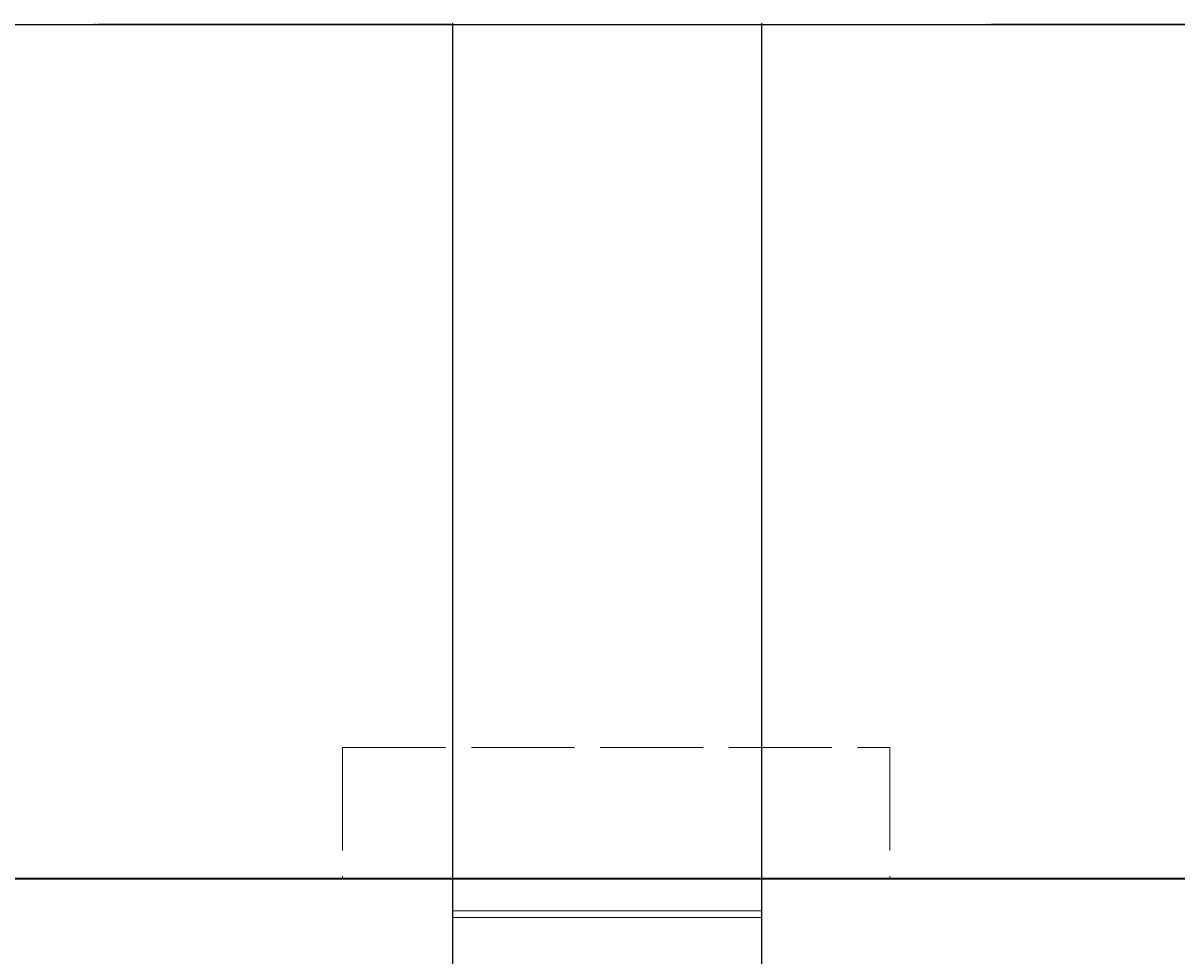
# Model space of a CAD drawing. Units: inches. Extents: x -61 to 1599, y -1316 to 257.
# Tile 153 of 204: x 406 to 540, y 149 to 257. Entities that reach past the tile are written whole.
import ezdxf

# ---------------------------------------------------------------- set-up
doc = ezdxf.new("R2010")
doc.units = ezdxf.units.IN
doc.header["$MEASUREMENT"] = 0
doc.linetypes.add('ACAD_ISO02W100', pattern=[15, 12, -3])
for name, color, linetype, lineweight in [('A-ANNO-DIMS', 2, 'Continuous', 18), ('A-FLOR-OVHD', 203, 'ACAD_ISO02W100', 13), ('WALLS', 4, 'Continuous', 35), ('WINDOWS', 220, 'Continuous', 18)]:
    doc.layers.add(name, color=color, linetype=linetype, lineweight=lineweight)
doc.styles.get("Standard").update_dxf_attribs({"font": 'arial.ttf'})
doc.dimstyles.get("Standard").update_dxf_attribs({"dimtxt": 0.18, "dimasz": 0.18, "dimexe": 0.18, "dimexo": 0.0625, "dimgap": 0.09, "dimtad": 0, "dimtih": 1, "dimtoh": 1, "dimdec": 0, "dimzin": 0, "dimdsep": 46, "dimlunit": 3, "dimtxsty": 'Standard', "dimcen": 0.09, "dimadec": 0, "dimazin": 0, "dimtfac": 1, "dimtdec": 0, "dimtofl": 0, "dimtmove": 0, "dimatfit": 3, "dimfxl": 1, "dimtolj": 1, "dimtzin": 0, "dimarcsym": 0})

# ---------------------------------------------------------------- blocks, each defined once
blk = doc.blocks.new('WIN-36IN')
for p, q in [((0, 4.5), (0, 9)), ((0, 9), (0, 0)), ((36, 9), (36, 0)), ((0, 5.26), (36, 5.26)), ((0, 4.5), (36, 4.5)), ((0, 4.5), (36, 4.5))]:
    blk.add_line(p, q)
blk = doc.blocks.new('*D686')
at = {"layer": 'A-ANNO-DIMS', "color": 0, "lineweight": -2, "transparency": 16777216}
for p, q in [((14.7, 157.74), (14.7, 257.46)), ((14.88, 257.28), (768.35, 257.28)), ((1522.52, 257.28), (769.05, 257.28)), ((1522.7, 157.74), (1522.7, 257.46))]:
    blk.add_line(p, q, dxfattribs=at)
at = {"layer": 'A-ANNO-DIMS', "color": 0, "transparency": 16777216}
for points in [[(14.88, 257.31), (14.88, 257.25), (14.7, 257.28)], [(1522.52, 257.31), (1522.52, 257.25), (1522.7, 257.28)]]:
    blk.add_solid(points, dxfattribs=at)
at = {"layer": 'DEFPOINTS', "color": 0, "transparency": 16777216}
for p in [(1522.7, 257.28), (14.7, 157.68), (1522.7, 157.68)]:
    blk.add_point(p, dxfattribs=at)
at = {"layer": 'A-ANNO-DIMS', "color": 0, "transparency": 16777216, "insert": (768.7, 257.28), "char_height": 0.18, "attachment_point": 5}
blk.add_mtext('\\A1;1508', dxfattribs=at)
blk = doc.blocks.new('*D703')
at = {"layer": 'A-ANNO-DIMS', "color": 0, "lineweight": -2, "transparency": 16777216}
for p, q in [((372.32, -616.88), (372.32, 257.46)), ((372.5, 257.28), (413.7, 257.28)), ((455.65, 257.28), (414.45, 257.28)), ((455.83, -616.88), (455.83, 257.46))]:
    blk.add_line(p, q, dxfattribs=at)
at = {"layer": 'A-ANNO-DIMS', "color": 0, "transparency": 16777216}
for points in [[(372.5, 257.31), (372.5, 257.25), (372.32, 257.28)], [(455.65, 257.31), (455.65, 257.25), (455.83, 257.28)]]:
    blk.add_solid(points, dxfattribs=at)
at = {"layer": 'DEFPOINTS', "color": 0, "transparency": 16777216}
for p in [(455.83, 257.28), (372.32, -616.94), (455.83, -616.94)]:
    blk.add_point(p, dxfattribs=at)
at = {"layer": 'A-ANNO-DIMS', "color": 0, "transparency": 16777216, "insert": (414.08, 257.28), "char_height": 0.18, "attachment_point": 5}
blk.add_mtext('\\A1;83.51', dxfattribs=at)
blk = doc.blocks.new('*D704')
at = {"layer": 'A-ANNO-DIMS', "color": 0, "lineweight": -2, "transparency": 16777216}
for p, q in [((491.83, -616.88), (491.83, 257.46)), ((492.01, 257.28), (517.87, 257.28)), ((544.52, 257.28), (518.66, 257.28)), ((544.7, -616.88), (544.7, 257.46))]:
    blk.add_line(p, q, dxfattribs=at)
at = {"layer": 'A-ANNO-DIMS', "color": 0, "transparency": 16777216}
for points in [[(492.01, 257.31), (492.01, 257.25), (491.83, 257.28)], [(544.52, 257.31), (544.52, 257.25), (544.7, 257.28)]]:
    blk.add_solid(points, dxfattribs=at)
at = {"layer": 'DEFPOINTS', "color": 0, "transparency": 16777216}
for p in [(544.7, 257.28), (491.83, -616.94), (544.7, -616.94)]:
    blk.add_point(p, dxfattribs=at)
at = {"layer": 'A-ANNO-DIMS', "color": 0, "transparency": 16777216, "insert": (518.27, 257.28), "char_height": 0.18, "attachment_point": 5}
blk.add_mtext('\\A1;52.87', dxfattribs=at)

msp = doc.modelspace()

# ---------------------------------------------------------------- linework, layer by layer
at = {"layer": 'A-FLOR-OVHD'}
for p, q in [((442.9886, 172.9695), (442.9886, 157.6771)), ((442.9886, 172.9695), (506.76, 172.9695)), ((506.76, 172.9695), (506.76, 157.6771))]:
    msp.add_line(p, q, dxfattribs=at)
at = {"layer": 'WALLS'}
msp.add_line((544.7028, 157.6771), (14.7028, 157.6771), dxfattribs=at)

# ---------------------------------------------------------------- block references
at = {"layer": 'WINDOWS'}
msp.add_blockref('WIN-36IN', (455.8326, 148.677), dxfattribs=at)

# ---------------------------------------------------------------- dimensions: what is measured, and where the dimension line sits
at = {"layer": 'A-ANNO-DIMS'}
for base, p1, p2, override, picture, middle in [((1522.7028, 257.2771), (14.7028, 157.6771), (1522.7028, 157.6771), {"dimdec": 0, "dimlfac": 1, "dimrnd": 0, "dimzin": 0, "dimdsep": 46, "dimlunit": 2}, '*D686', (768.7028, 257.2771)), ((455.8327, 257.2771), (372.3201, -616.9446), (455.8327, -616.9446), {"dimdec": 2, "dimlfac": 1, "dimrnd": 0, "dimzin": 0, "dimdsep": 46, "dimlunit": 2}, '*D703', (414.0764, 257.2771)), ((544.7028, 257.2771), (491.8327, -616.9446), (544.7028, -616.9446), {"dimdec": 2, "dimlfac": 1, "dimrnd": 0, "dimzin": 0, "dimdsep": 46, "dimlunit": 2}, '*D704', (518.2677, 257.2771))]:
    dim = msp.add_linear_dim(base=base, p1=p1, p2=p2, dimstyle='Standard', override=override, dxfattribs=at)
    dim.commit()
    dim.dimension.update_dxf_attribs({"geometry": picture, "text_midpoint": middle})

doc.saveas('drawing.dxf')
